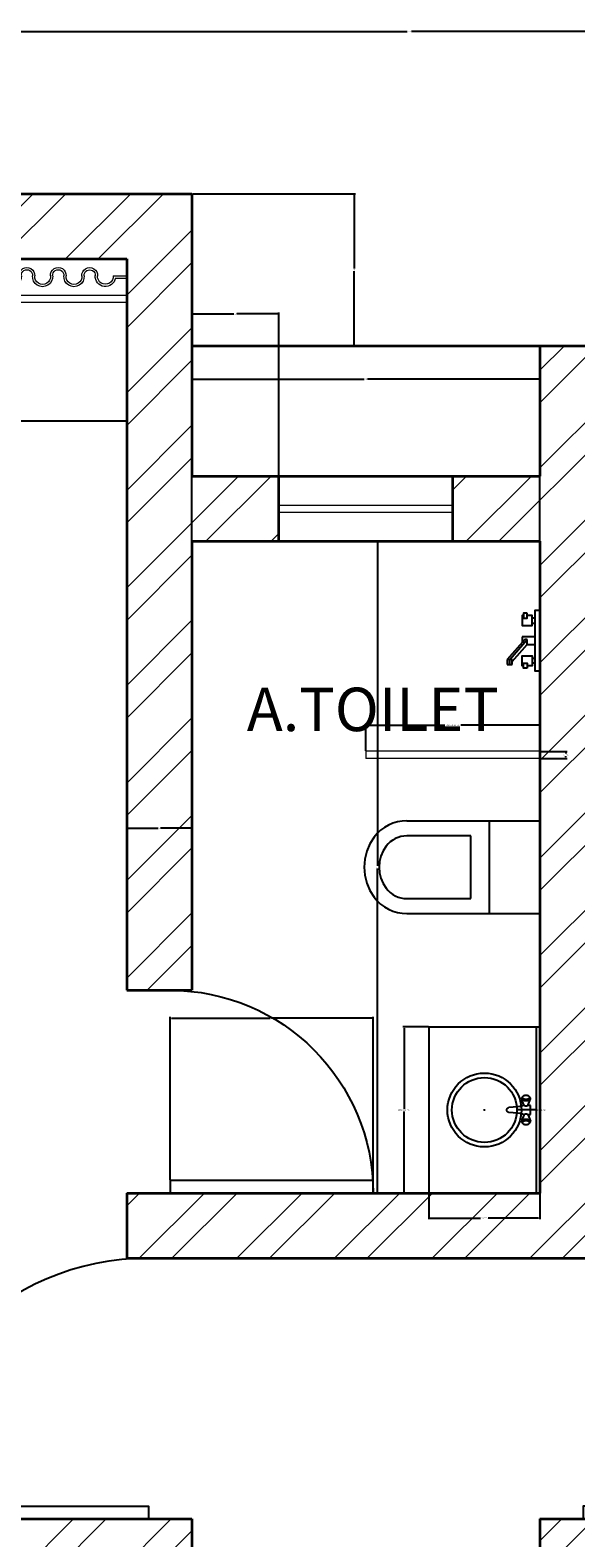
# Model space of a CAD drawing. Units: inches. Extents: x 3449 to 3843, y 1566 to 2054.
# Tile 7 of 8: x 3594 to 3669, y 1846 to 2054. Entities that reach past the tile are written whole.
import ezdxf

# ---------------------------------------------------------------- set-up
doc = ezdxf.new("R2010")
doc.units = ezdxf.units.IN
for name, color, linetype, lineweight in [('A-ANNO-DIMS', 2, 'Continuous', 18), ('A-AREA-IDEN', 7, 'Continuous', 25), ('A-DOOR', 4, 'Continuous', 25), ('A-FURN-DRAP', 32, 'Continuous', 13), ('A-GLAZ', 5, 'Continuous', 18), ('A-WALL', 7, 'Continuous', 35), ('A-WALL-PATT', 251, 'Continuous', 13), ('Сантехника', 7, 'Continuous', 18)]:
    doc.layers.add(name, color=color, linetype=linetype, lineweight=lineweight)
doc.layers.add('SANTEH', color=7, linetype='Continuous')
doc.styles.get("Standard").update_dxf_attribs({"font": 'arial.ttf'})
doc.dimstyles.get("Standard").update_dxf_attribs({"dimtxt": 0.18, "dimasz": 0.18, "dimexe": 0.18, "dimexo": 0.0625, "dimgap": 0.09, "dimtad": 0, "dimtih": 1, "dimtoh": 1, "dimdec": 4, "dimzin": 0, "dimdsep": 46, "dimtxsty": 'Standard', "dimcen": 0.09, "dimadec": 0, "dimazin": 0, "dimtfac": 1, "dimtdec": 4, "dimtofl": 0, "dimtmove": 0, "dimatfit": 3, "dimfxl": 1, "dimtolj": 1, "dimtzin": 0, "dimarcsym": 0})

# ---------------------------------------------------------------- blocks, each defined once
blk = doc.blocks.new('*U5')
for p, q in [((0, 0), (0, -6)), ((36, 0), (36, -6))]:
    blk.add_line(p, q)
blk.add_lwpolyline([(0, 0), (0, 36), (1.75, 36), (1.75, 0)], close=True)
blk.add_arc((0, 0), 36, 0, 90)
blk = doc.blocks.new('*U7')
for p, q in [((0, 0), (0, -6)), ((28, 0), (28, -6))]:
    blk.add_line(p, q)
blk.add_lwpolyline([(0, 0), (0, 28), (1.75, 28), (1.75, 0)], close=True)
blk.add_arc((0, 0), 28, 0, 90)
blk = doc.blocks.new('Basin Built-In Circle_74')
at = {"layer": 'SANTEH'}
for p, q in [((0, 600), (900, 600)), ((0, 0), (0, 600)), ((0, 580), (900, 580)), ((900, 0), (900, 600)), ((371.7, 528.5), (371.5, 525)), ((371.7, 528.5), (371.5, 525)), ((371.5, 525), (371.7, 521.5)), ((371.5, 525), (371.7, 521.5)), ((372.1, 531.8), (371.7, 528.5)), ((372.1, 531.8), (371.7, 528.5)), ((371.7, 521.5), (372.1, 518.2)), ((371.7, 521.5), (372.1, 518.2)), ((372.8, 535), (372.1, 531.8)), ((372.8, 535), (372.1, 531.8)), ((372.1, 518.2), (372.8, 515)), ((372.1, 518.2), (372.8, 515)), ((373.8, 537.9), (372.8, 535)), ((373.8, 537.9), (372.8, 535)), ((372.8, 515), (373.8, 512.1)), ((372.8, 515), (373.8, 512.1)), ((375.1, 540.3), (373.8, 537.9)), ((375.1, 540.3), (373.8, 537.9)), ((373.8, 512.1), (375.1, 509.7)), ((373.8, 512.1), (375.1, 509.7)), ((376.5, 542.3), (375.1, 540.3)), ((376.5, 542.3), (375.1, 540.3)), ((375.1, 509.7), (376.5, 507.7)), ((375.1, 509.7), (376.5, 507.7)), ((378.1, 543.8), (376.5, 542.3)), ((378.1, 543.8), (376.5, 542.3)), ((376.5, 507.7), (378.1, 506.2)), ((376.5, 507.7), (378.1, 506.2)), ((382.6, 547.6), (378.1, 543.8)), ((382.6, 547.6), (378.1, 543.8)), ((379.8, 544.7), (378.1, 543.8)), ((379.8, 544.7), (378.1, 543.8)), ((378.1, 506.2), (379.8, 505.3)), ((382.6, 502.4), (378.1, 506.2)), ((378.1, 506.2), (379.8, 505.3)), ((382.6, 502.4), (378.1, 506.2)), ((381.5, 545), (379.8, 544.7)), ((381.5, 545), (379.8, 544.7)), ((379.8, 505.3), (381.5, 505)), ((379.8, 505.3), (381.5, 505)), ((383.2, 544.7), (381.5, 545)), ((383.2, 544.7), (381.5, 545)), ((381.5, 505), (383.2, 505.3)), ((381.5, 505), (383.2, 505.3)), ((384.6, 548.6), (382.6, 547.6)), ((384.6, 548.6), (382.6, 547.6)), ((382.6, 502.4), (384.6, 501.4)), ((382.6, 502.4), (384.6, 501.4)), ((384.9, 543.8), (383.2, 544.7)), ((384.9, 543.8), (383.2, 544.7)), ((383.2, 505.3), (384.9, 506.2)), ((383.2, 505.3), (384.9, 506.2)), ((386.7, 549), (384.6, 548.6)), ((386.7, 549), (384.6, 548.6)), ((384.6, 501.4), (386.7, 501)), ((384.6, 501.4), (386.7, 501)), ((386.5, 542.3), (384.9, 543.8)), ((386.5, 542.3), (384.9, 543.8)), ((384.9, 506.2), (386.5, 507.7)), ((384.9, 506.2), (386.5, 507.7)), ((387.9, 540.3), (386.5, 542.3)), ((387.9, 540.3), (386.5, 542.3)), ((386.5, 507.7), (387.9, 509.7)), ((386.5, 507.7), (387.9, 509.7)), ((388.8, 548.6), (386.7, 549)), ((388.8, 548.6), (386.7, 549)), ((386.7, 501), (388.8, 501.4)), ((386.7, 501), (388.8, 501.4)), ((389.2, 537.9), (387.9, 540.3)), ((389.2, 537.9), (387.9, 540.3)), ((387.9, 509.7), (389.2, 512.1)), ((387.9, 509.7), (389.2, 512.1)), ((390.8, 547.6), (388.8, 548.6)), ((422.4, 536.8), (388.8, 548.6)), ((390.8, 547.6), (388.8, 548.6)), ((422.4, 536.8), (388.8, 548.6)), ((422.4, 513.2), (388.8, 501.4)), ((422.4, 513.2), (388.8, 501.4)), ((388.8, 501.4), (390.8, 502.4)), ((388.8, 501.4), (390.8, 502.4)), ((390.2, 535), (389.2, 537.9)), ((390.2, 535), (389.2, 537.9)), ((389.2, 512.1), (390.2, 515)), ((389.2, 512.1), (390.2, 515)), ((390.9, 531.8), (390.2, 535)), ((390.9, 531.8), (390.2, 535)), ((390.2, 515), (390.9, 518.2)), ((390.2, 515), (390.9, 518.2)), ((392.7, 545.8), (390.8, 547.6)), ((392.7, 545.8), (390.8, 547.6)), ((390.8, 502.4), (392.7, 504.2)), ((390.8, 502.4), (392.7, 504.2)), ((391.4, 528.5), (390.9, 531.8)), ((391.4, 528.5), (390.9, 531.8)), ((390.9, 518.2), (391.4, 521.5)), ((390.9, 518.2), (391.4, 521.5)), ((391.5, 525), (391.4, 528.5)), ((391.5, 525), (391.4, 528.5)), ((391.4, 521.5), (391.5, 525)), ((391.4, 521.5), (391.5, 525)), ((394.4, 543.4), (392.7, 545.8)), ((394.4, 543.4), (392.7, 545.8)), ((392.7, 504.2), (394.4, 506.6)), ((392.7, 504.2), (394.4, 506.6)), ((395.9, 540.4), (394.4, 543.4)), ((395.9, 540.4), (394.4, 543.4)), ((394.4, 506.6), (395.9, 509.6)), ((394.4, 506.6), (395.9, 509.6)), ((397.1, 537), (395.9, 540.4)), ((397.1, 537), (395.9, 540.4)), ((395.9, 509.6), (397.1, 513)), ((395.9, 509.6), (397.1, 513)), ((398, 533.2), (397.1, 537)), ((398, 533.2), (397.1, 537)), ((397.1, 513), (398, 516.8)), ((397.1, 513), (398, 516.8)), ((398.5, 529.2), (398, 533.2)), ((398.5, 529.2), (398, 533.2)), ((398, 516.8), (398.5, 520.8)), ((398, 516.8), (398.5, 520.8)), ((398.7, 525), (398.5, 529.2)), ((398.7, 525), (398.5, 529.2)), ((398.5, 520.8), (398.7, 525)), ((398.5, 520.8), (398.7, 525)), ((423.4, 536.3), (422.4, 536.8)), ((423.4, 536.3), (422.4, 536.8)), ((422.4, 513.2), (423.4, 513.7)), ((422.4, 513.2), (423.4, 513.7)), ((424.3, 535.4), (423.4, 536.3)), ((424.3, 535.4), (423.4, 536.3)), ((423.4, 513.7), (424.3, 514.6)), ((423.4, 513.7), (424.3, 514.6)), ((425.2, 534.2), (424.3, 535.4)), ((425.2, 534.2), (424.3, 535.4)), ((424.3, 514.6), (425.2, 515.8)), ((424.3, 514.6), (425.2, 515.8)), ((426.7, 535), (424.6, 535)), ((426.7, 535), (424.6, 535)), ((427.1, 515), (424.6, 515)), ((427.1, 515), (424.6, 515)), ((425.2, 548), (425, 547.5)), ((425.2, 548), (425, 547.5)), ((425, 547.5), (425, 547)), ((425, 547.5), (425, 547)), ((425, 547), (425, 535)), ((425, 547), (425, 535)), ((425, 515), (425, 513)), ((425, 515), (425, 513)), ((425, 513), (425, 512.5)), ((425, 513), (425, 512.5)), ((425, 512.5), (425.2, 512)), ((425, 512.5), (425.2, 512)), ((425.4, 548.5), (425.2, 548)), ((425.4, 548.5), (425.2, 548)), ((425.9, 532.7), (425.2, 534.2)), ((425.9, 532.7), (425.2, 534.2)), ((425.2, 515.8), (425.9, 517.3)), ((425.2, 515.8), (425.9, 517.3)), ((425.2, 512), (428.1, 505.1)), ((425.2, 512), (428.1, 505.1)), ((425.7, 548.9), (425.4, 548.5)), ((425.7, 548.9), (425.4, 548.5)), ((426.1, 549.3), (425.7, 548.9)), ((426.1, 549.3), (425.7, 548.9)), ((426.5, 531), (425.9, 532.7)), ((426.5, 531), (425.9, 532.7)), ((425.9, 517.3), (426.5, 519)), ((425.9, 517.3), (426.5, 519)), ((426.5, 549.6), (426.1, 549.3)), ((426.5, 549.6), (426.1, 549.3)), ((427, 549.8), (426.5, 549.6)), ((427, 549.8), (426.5, 549.6)), ((427, 529.1), (426.5, 531)), ((427, 529.1), (426.5, 531)), ((426.5, 519), (427, 520.9)), ((426.5, 519), (427, 520.9)), ((427.5, 550), (427, 549.8)), ((427.5, 550), (427, 549.8)), ((427.2, 527.1), (427, 529.1)), ((427.2, 527.1), (427, 529.1)), ((427, 520.9), (427.2, 522.9)), ((427, 520.9), (427.2, 522.9)), ((427.3, 525), (427.2, 527.1)), ((427.3, 525), (427.2, 527.1)), ((427.2, 522.9), (427.3, 525)), ((427.2, 522.9), (427.3, 525)), ((428, 550), (427.5, 550)), ((428, 550), (427.5, 550)), ((472, 550), (428, 550)), ((472, 550), (428, 550)), ((428, 505.4), (430.7, 493.4)), ((428, 505.4), (430.7, 493.4)), ((430.7, 493.4), (433, 477.1)), ((430.7, 493.4), (433, 477.1)), ((469.3, 493.4), (467, 477.1)), ((469.3, 493.4), (467, 477.1)), ((472, 505.4), (469.3, 493.4)), ((472, 505.4), (469.3, 493.4)), ((474.8, 512), (471.9, 505.1)), ((474.8, 512), (471.9, 505.1)), ((472.5, 550), (472, 550)), ((472.5, 550), (472, 550)), ((473, 549.8), (472.5, 550)), ((473, 549.8), (472.5, 550)), ((472.8, 527.1), (472.7, 525)), ((472.8, 527.1), (472.7, 525)), ((472.7, 525), (472.8, 522.9)), ((472.7, 525), (472.8, 522.9)), ((473, 529.1), (472.8, 527.1)), ((473, 529.1), (472.8, 527.1)), ((472.8, 522.9), (473, 520.9)), ((472.8, 522.9), (473, 520.9)), ((473.5, 549.6), (473, 549.8)), ((473.5, 549.6), (473, 549.8)), ((473.5, 531), (473, 529.1)), ((473.5, 531), (473, 529.1)), ((473, 520.9), (473.5, 519)), ((473, 520.9), (473.5, 519)), ((475.4, 515), (473.2, 515)), ((475.4, 515), (473.2, 515)), ((473.9, 549.3), (473.5, 549.6)), ((473.9, 549.3), (473.5, 549.6)), ((475.4, 535), (473.5, 535)), ((475.4, 535), (473.5, 535)), ((474.1, 532.7), (473.5, 531)), ((474.1, 532.7), (473.5, 531)), ((473.5, 519), (474.1, 517.3)), ((473.5, 519), (474.1, 517.3)), ((474.3, 548.9), (473.9, 549.3)), ((474.3, 548.9), (473.9, 549.3)), ((474.8, 534.2), (474.1, 532.7)), ((474.8, 534.2), (474.1, 532.7)), ((474.1, 517.3), (474.8, 515.8)), ((474.1, 517.3), (474.8, 515.8)), ((474.6, 548.5), (474.3, 548.9)), ((474.6, 548.5), (474.3, 548.9)), ((474.8, 548), (474.6, 548.5)), ((474.8, 548), (474.6, 548.5)), ((475, 547.5), (474.8, 548)), ((475, 547.5), (474.8, 548)), ((475.7, 535.4), (474.8, 534.2)), ((475.7, 535.4), (474.8, 534.2)), ((474.8, 515.8), (475.7, 514.6)), ((474.8, 515.8), (475.7, 514.6)), ((474.8, 512), (475, 512.5)), ((474.8, 512), (475, 512.5)), ((475, 547), (475, 547.5)), ((475, 547), (475, 547.5)), ((475, 535), (475, 547)), ((475, 535), (475, 547)), ((475, 513), (475, 515)), ((475, 513), (475, 515)), ((475, 512.5), (475, 513)), ((475, 512.5), (475, 513)), ((476.6, 536.3), (475.7, 535.4)), ((476.6, 536.3), (475.7, 535.4)), ((475.7, 514.6), (476.6, 513.7)), ((475.7, 514.6), (476.6, 513.7)), ((477.6, 536.8), (476.6, 536.3)), ((477.6, 536.8), (476.6, 536.3)), ((476.6, 513.7), (477.6, 513.2)), ((476.6, 513.7), (477.6, 513.2)), ((477.6, 536.8), (511.2, 548.6)), ((477.6, 536.8), (511.2, 548.6)), ((477.6, 513.2), (511.2, 501.4)), ((477.6, 513.2), (511.2, 501.4)), ((501.5, 529.2), (501.3, 525)), ((501.5, 529.2), (501.3, 525)), ((501.3, 525), (501.5, 520.8)), ((501.3, 525), (501.5, 520.8)), ((502, 533.2), (501.5, 529.2)), ((502, 533.2), (501.5, 529.2)), ((501.5, 520.8), (502, 516.8)), ((501.5, 520.8), (502, 516.8)), ((502.9, 537), (502, 533.2)), ((502.9, 537), (502, 533.2)), ((502, 516.8), (502.9, 513)), ((502, 516.8), (502.9, 513)), ((504.1, 540.4), (502.9, 537)), ((504.1, 540.4), (502.9, 537)), ((502.9, 513), (504.1, 509.6)), ((502.9, 513), (504.1, 509.6)), ((505.6, 543.4), (504.1, 540.4)), ((505.6, 543.4), (504.1, 540.4)), ((504.1, 509.6), (505.6, 506.6)), ((504.1, 509.6), (505.6, 506.6)), ((507.3, 545.8), (505.6, 543.4)), ((507.3, 545.8), (505.6, 543.4)), ((505.6, 506.6), (507.3, 504.2)), ((505.6, 506.6), (507.3, 504.2)), ((509.2, 547.6), (507.3, 545.8)), ((509.2, 547.6), (507.3, 545.8)), ((507.3, 504.2), (509.2, 502.4)), ((507.3, 504.2), (509.2, 502.4)), ((508.6, 528.5), (508.5, 525)), ((508.6, 528.5), (508.5, 525)), ((508.5, 525), (508.6, 521.5)), ((508.5, 525), (508.6, 521.5)), ((509.1, 531.8), (508.6, 528.5)), ((509.1, 531.8), (508.6, 528.5)), ((508.6, 521.5), (509.1, 518.2)), ((508.6, 521.5), (509.1, 518.2)), ((509.8, 535), (509.1, 531.8)), ((509.8, 535), (509.1, 531.8)), ((509.1, 518.2), (509.8, 515)), ((509.1, 518.2), (509.8, 515)), ((511.2, 548.6), (509.2, 547.6)), ((511.2, 548.6), (509.2, 547.6)), ((509.2, 502.4), (511.2, 501.4)), ((509.2, 502.4), (511.2, 501.4)), ((510.8, 537.9), (509.8, 535)), ((510.8, 537.9), (509.8, 535)), ((509.8, 515), (510.8, 512.1)), ((509.8, 515), (510.8, 512.1)), ((512.1, 540.3), (510.8, 537.9)), ((512.1, 540.3), (510.8, 537.9)), ((510.8, 512.1), (512.1, 509.7)), ((510.8, 512.1), (512.1, 509.7)), ((513.3, 549), (511.2, 548.6)), ((513.3, 549), (511.2, 548.6)), ((511.2, 501.4), (513.3, 501)), ((511.2, 501.4), (513.3, 501)), ((513.5, 542.3), (512.1, 540.3)), ((513.5, 542.3), (512.1, 540.3)), ((512.1, 509.7), (513.5, 507.7)), ((512.1, 509.7), (513.5, 507.7)), ((515.4, 548.6), (513.3, 549)), ((515.4, 548.6), (513.3, 549)), ((513.3, 501), (515.4, 501.4)), ((513.3, 501), (515.4, 501.4)), ((515.1, 543.8), (513.5, 542.3)), ((515.1, 543.8), (513.5, 542.3)), ((513.5, 507.7), (515.1, 506.2)), ((513.5, 507.7), (515.1, 506.2)), ((516.8, 544.7), (515.1, 543.8)), ((516.8, 544.7), (515.1, 543.8)), ((515.1, 506.2), (516.8, 505.3)), ((515.1, 506.2), (516.8, 505.3)), ((517.4, 547.6), (515.4, 548.6)), ((517.4, 547.6), (515.4, 548.6)), ((515.4, 501.4), (517.4, 502.4)), ((515.4, 501.4), (517.4, 502.4)), ((518.5, 545), (516.8, 544.7)), ((518.5, 545), (516.8, 544.7)), ((516.8, 505.3), (518.5, 505)), ((516.8, 505.3), (518.5, 505)), ((517.4, 547.6), (521.9, 543.8)), ((517.4, 547.6), (521.9, 543.8)), ((517.4, 502.4), (521.9, 506.2)), ((517.4, 502.4), (521.9, 506.2)), ((520.2, 544.7), (518.5, 545)), ((520.2, 544.7), (518.5, 545)), ((518.5, 505), (520.2, 505.3)), ((518.5, 505), (520.2, 505.3)), ((521.9, 543.8), (520.2, 544.7)), ((521.9, 543.8), (520.2, 544.7)), ((520.2, 505.3), (521.9, 506.2)), ((520.2, 505.3), (521.9, 506.2)), ((523.5, 542.3), (521.9, 543.8)), ((523.5, 542.3), (521.9, 543.8)), ((521.9, 506.2), (523.5, 507.7)), ((521.9, 506.2), (523.5, 507.7)), ((524.9, 540.3), (523.5, 542.3)), ((524.9, 540.3), (523.5, 542.3)), ((523.5, 507.7), (524.9, 509.7)), ((523.5, 507.7), (524.9, 509.7)), ((526.2, 537.9), (524.9, 540.3)), ((526.2, 537.9), (524.9, 540.3)), ((524.9, 509.7), (526.2, 512.1)), ((524.9, 509.7), (526.2, 512.1)), ((527.2, 535), (526.2, 537.9)), ((527.2, 535), (526.2, 537.9)), ((526.2, 512.1), (527.2, 515)), ((526.2, 512.1), (527.2, 515)), ((527.9, 531.8), (527.2, 535)), ((527.9, 531.8), (527.2, 535)), ((527.2, 515), (527.9, 518.2)), ((527.2, 515), (527.9, 518.2)), ((528.3, 528.5), (527.9, 531.8)), ((528.3, 528.5), (527.9, 531.8)), ((527.9, 518.2), (528.3, 521.5)), ((527.9, 518.2), (528.3, 521.5)), ((528.5, 525), (528.3, 528.5)), ((528.5, 525), (528.3, 528.5)), ((528.3, 521.5), (528.5, 525)), ((528.3, 521.5), (528.5, 525)), ((433, 477.2), (435, 456.1)), ((433, 477.2), (435, 456.1)), ((435, 456.1), (436.8, 432.9)), ((435, 456.1), (436.8, 432.9)), ((437, 430.8), (436.8, 432.9)), ((437, 430.8), (436.8, 432.9)), ((437, 430.7), (437, 430.8)), ((437, 430.7), (437, 430.8)), ((437.6, 428.7), (437, 430.7)), ((437.6, 428.7), (437, 430.7)), ((438.6, 426.9), (437.6, 428.7)), ((438.6, 426.9), (437.6, 428.7)), ((440, 425.1), (438.6, 426.9)), ((440, 425.1), (438.6, 426.9)), ((441.6, 423.7), (440, 425.1)), ((441.6, 423.7), (440, 425.1)), ((443.5, 422.5), (441.6, 423.7)), ((443.5, 422.5), (441.6, 423.7)), ((445.6, 421.7), (443.5, 422.5)), ((445.6, 421.7), (443.5, 422.5)), ((445, 421.7), (443.9, 422.4)), ((446.6, 421), (445, 421.7)), ((447.7, 421.2), (445.6, 421.7)), ((447.7, 421.2), (445.6, 421.7)), ((448.3, 420.6), (446.6, 421)), ((450, 421), (447.7, 421.2)), ((450, 421), (447.7, 421.2)), ((450, 420.5), (448.3, 420.6)), ((452.3, 421.2), (450, 421)), ((452.3, 421.2), (450, 421)), ((451.7, 420.6), (450, 420.5)), ((453.4, 421), (451.7, 420.6)), ((454.4, 421.7), (452.3, 421.2)), ((454.4, 421.7), (452.3, 421.2)), ((455, 421.7), (453.4, 421)), ((456.5, 422.5), (454.4, 421.7)), ((456.5, 422.5), (454.4, 421.7)), ((456.1, 422.4), (455, 421.7)), ((458.4, 423.7), (456.5, 422.5)), ((458.4, 423.7), (456.5, 422.5)), ((460, 425.1), (458.4, 423.7)), ((460, 425.1), (458.4, 423.7)), ((461.4, 426.9), (460, 425.1)), ((461.4, 426.9), (460, 425.1)), ((462.4, 428.7), (461.4, 426.9)), ((462.4, 428.7), (461.4, 426.9)), ((463, 430.7), (462.4, 428.7)), ((463, 430.7), (462.4, 428.7)), ((463.2, 432.9), (463, 430.8)), ((463.2, 432.9), (463, 430.8)), ((463, 430.7), (463, 430.8)), ((463, 430.7), (463, 430.8)), ((465, 456.1), (463.2, 432.9)), ((465, 456.1), (463.2, 432.9)), ((467, 477.2), (465, 456.1)), ((467, 477.2), (465, 456.1)), ((0, 0), (900, 0))]:
    blk.add_line(p, q, dxfattribs=at)
for radius in [200, 175.8]:
    blk.add_circle((450, 300), radius, dxfattribs=at)
blk = doc.blocks.new('WC With Cistern_103')
at = {"layer": 'SANTEH'}
for p, q in [((0, 170), (0, 700)), ((370, 700), (0, 700)), ((370, 170), (370, 700)), ((370, 500), (0, 500)), ((60, 425), (60, 170)), ((310, 425), (60, 425)), ((310, 170), (310, 425))]:
    blk.add_line(p, q, dxfattribs=at)
for points in [[(0, 170), (1.1, 151.2), (4.3, 132.7), (9.7, 114.6), (17.1, 97.3), (26.5, 81), (37.7, 65.9), (50.6, 52.1), (65, 40)], [(60, 170), (60.7, 158.1), (62.7, 146.5), (66.1, 135.1), (70.8, 124.2), (76.7, 113.9), (83.8, 104.3), (91.9, 95.7), (101, 88)], [(269, 88), (278.1, 95.7), (286.2, 104.3), (293.3, 113.9), (299.2, 124.2), (303.9, 135.1), (307.3, 146.5), (309.3, 158.1), (310, 170)], [(305, 40), (319.4, 52.1), (332.3, 65.9), (343.5, 81), (352.9, 97.3), (360.3, 114.6), (365.7, 132.7), (368.9, 151.2), (370, 170)], [(101, 88), (120, 76), (140.7, 67.2), (162.6, 61.8), (185, 60), (207.4, 61.8), (229.3, 67.2), (250, 76), (269, 88)], [(65, 40), (92.2, 22.8), (121.8, 10.3), (153, 2.6), (185, 0), (217, 2.6), (248.2, 10.3), (277.8, 22.8), (305, 40)]]:
    blk.add_lwpolyline(points, dxfattribs=at)
blk = doc.blocks.new('Faucet - kit sink front')
at = {"layer": 'SANTEH'}
for p, q in [((-0.25, 3), (3.75, 6.5)), ((3.75, 6), (3.75, 6.5)), ((3.75, 6.5), (4.75, 6.5)), ((4.75, 6.5), (4.75, 6)), ((-0.75, 3.5), (0.3192, 3.5)), ((-0.75, 1), (-0.75, 3.5)), ((3.75, 6), (-0.25, 2.5)), ((4.1921, 5.5041), (0.75, 2.5)), ((3.75, 5.5), (3.75, 6)), ((4.75, 6), (3.75, 6)), ((4.75, 5.5), (3.75, 5.5)), ((4.75, 6), (4.75, 5.5)), ((-4.5, 1), (-4.5, 1.5)), ((-3.5, 1.5), (-3.5, 1)), ((-0.25, 2.5), (-0.25, 3)), ((0.75, 2.5), (-0.25, 2.5)), ((0.75, 2.5), (0.75, 1)), ((3.5, 1.5), (3.5, 1)), ((4.5, 1), (4.5, 1.5))]:
    blk.add_line(p, q, dxfattribs=at)
for points in [[(-5.5, 2.5), (-5.5, 3.25), (-4.5, 3.25), (-4.5, 2.5)], [(5.5, 2.5), (5.5, 3.25), (4.5, 3.25), (4.5, 2.5)], [(-6, 0), (-6, 1), (6, 1), (6, 0)]]:
    blk.add_lwpolyline(points, close=True, dxfattribs=at)
for points in [[(-5, 3.2513), (-5, 3.5), (-3, 3.5), (-3, 1.5), (-5, 1.5), (-5, 2.5)], [(5, 3.2513), (5, 3.5), (3, 3.5), (3, 1.5), (5, 1.5), (5, 2.5)]]:
    blk.add_lwpolyline(points, dxfattribs=at)
blk = doc.blocks.new('DRAPERY-PANEL')
for p, q in [((1.19, 47.95), (1.19, 49.52)), ((1.5, 47.66), (1.5, 49.52))]:
    blk.add_line(p, q)
for centre, radius, start, end in [((1.42, 46.57), 1.4, 99.481, 274.2422), ((1.42, 46.57), 1.09, 85.7578, 274.2422), ((1.55, 44.41), 1.09, 265.7578, 94.2422), ((1.55, 44.41), 0.776, 265.7578, 94.2422), ((1.4, 42.24), 1.4, 85.7578, 274.2422), ((1.4, 42.24), 1.09, 85.7578, 274.2422), ((1.56, 40.07), 1.09, 265.7578, 94.2422), ((1.56, 40.07), 0.776, 265.7578, 94.2422), ((1.4, 37.91), 1.4, 85.7578, 274.2422), ((1.4, 37.91), 1.09, 85.7578, 274.2422), ((1.56, 35.74), 1.09, 265.7578, 94.2422), ((1.56, 35.74), 0.776, 265.7578, 94.2422), ((1.4, 33.58), 1.4, 85.7578, 274.2422), ((1.4, 33.58), 1.09, 85.7578, 274.2422), ((1.56, 31.41), 1.09, 265.7578, 94.2422), ((1.56, 31.41), 0.776, 265.7578, 94.2422), ((1.41, 29.24), 1.4, 85.7578, 274.2422), ((1.41, 29.24), 1.09, 85.7578, 274.2422), ((1.57, 27.08), 1.09, 265.7578, 94.2422), ((1.57, 27.08), 0.776, 265.7578, 94.2422), ((1.41, 24.91), 1.4, 85.7578, 274.2422), ((1.41, 24.91), 1.09, 85.7578, 274.2422), ((1.57, 22.74), 1.09, 265.7578, 94.2422), ((1.57, 22.74), 0.776, 265.7578, 94.2422), ((1.41, 20.58), 1.4, 85.7578, 274.2422), ((1.41, 20.58), 1.09, 85.7578, 274.2422), ((1.58, 18.41), 1.09, 265.7578, 94.2422), ((1.58, 18.41), 0.776, 265.7578, 94.2422), ((1.42, 16.25), 1.4, 85.7578, 274.2422), ((1.42, 16.25), 1.09, 85.7578, 274.2422), ((1.58, 14.08), 1.09, 265.7578, 94.2422), ((1.58, 14.08), 0.776, 265.7578, 94.2422), ((1.42, 11.91), 1.4, 85.7578, 274.2422), ((1.42, 11.91), 1.09, 85.7578, 274.2422), ((1.58, 9.75), 1.09, 265.7578, 94.2422), ((1.58, 9.75), 0.776, 265.7578, 94.2422), ((1.43, 7.58), 1.4, 85.7578, 274.2422), ((1.43, 7.58), 1.09, 85.7578, 274.2422), ((1.59, 5.42), 1.09, 265.7578, 94.2422), ((1.43, 3.25), 1.4, 85.7578, 274.2422), ((1.43, 3.25), 1.09, 85.7578, 274.2422), ((1.59, 5.42), 0.776, 265.7578, 94.2422), ((1.59, 1.08), 1.09, 265.7578, 94.2422), ((1.59, 1.08), 0.776, 265.7578, 94.2422)]:
    blk.add_arc(centre, radius, start, end)
blk = doc.blocks.new('SHOWER-SCREEN-24')
for p, q in [((0, 24), (0, 0)), ((1, 24), (1, 0)), ((0, 0), (1, 0))]:
    blk.add_line(p, q)
blk = doc.blocks.new('GLAZING-24')
for p, q in [((24, 1), (0, 1)), ((24, 0), (0, 0))]:
    blk.add_line(p, q)
blk = doc.blocks.new('*D48')
at = {"layer": 'A-ANNO-DIMS', "color": 0, "lineweight": -2, "transparency": 16777216}
for p, q in [((3648.73, 1916.56), (3645.17, 1916.56)), ((3645.35, 1916.38), (3645.35, 1905.27)), ((3645.35, 1893.79), (3645.35, 1904.9)), ((3648.73, 1893.61), (3645.17, 1893.61))]:
    blk.add_line(p, q, dxfattribs=at)
at = {"layer": 'A-ANNO-DIMS', "color": 0, "transparency": 16777216}
for points in [[(3645.32, 1916.38), (3645.38, 1916.38), (3645.35, 1916.56)], [(3645.32, 1893.79), (3645.38, 1893.79), (3645.35, 1893.61)]]:
    blk.add_solid(points, dxfattribs=at)
at = {"layer": 'Defpoints', "color": 0, "transparency": 16777216}
for p in [(3648.79, 1916.56), (3645.35, 1893.61), (3648.79, 1893.61)]:
    blk.add_point(p, dxfattribs=at)
at = {"layer": 'A-ANNO-DIMS', "color": 0, "transparency": 16777216, "insert": (3645.35, 1905.09), "char_height": 0.18, "attachment_point": 5}
blk.add_mtext('\\A1;BASIN 23 TYP.', dxfattribs=at)
blk = doc.blocks.new('*D49')
at = {"layer": 'A-ANNO-DIMS', "color": 0, "lineweight": -2, "transparency": 16777216}
for p, q in [((3648.79, 1893.55), (3648.79, 1889.99)), ((3664.09, 1893.55), (3664.09, 1889.99)), ((3648.97, 1890.17), (3655.92, 1890.17)), ((3663.91, 1890.17), (3656.96, 1890.17))]:
    blk.add_line(p, q, dxfattribs=at)
at = {"layer": 'A-ANNO-DIMS', "color": 0, "transparency": 16777216}
for points in [[(3648.97, 1890.2), (3648.97, 1890.14), (3648.79, 1890.17)], [(3663.91, 1890.2), (3663.91, 1890.14), (3664.09, 1890.17)]]:
    blk.add_solid(points, dxfattribs=at)
at = {"layer": 'Defpoints', "color": 0, "transparency": 16777216}
for p in [(3648.79, 1893.61), (3664.09, 1893.61), (3664.09, 1890.17)]:
    blk.add_point(p, dxfattribs=at)
at = {"layer": 'A-ANNO-DIMS', "color": 0, "transparency": 16777216, "insert": (3656.44, 1890.17), "char_height": 0.18, "attachment_point": 5}
blk.add_mtext('\\A1;15 TYP.', dxfattribs=at)
blk = doc.blocks.new('*D56')
at = {"layer": 'A-ANNO-DIMS', "color": 0, "lineweight": -2, "transparency": 16777216}
for p, q in [((3640.09, 1954.68), (3640.09, 1958.39)), ((3640.27, 1958.21), (3651, 1958.21)), ((3663.91, 1958.21), (3653.17, 1958.21)), ((3664.09, 1954.68), (3664.09, 1958.39))]:
    blk.add_line(p, q, dxfattribs=at)
at = {"layer": 'A-ANNO-DIMS', "color": 0, "transparency": 16777216}
for points in [[(3640.27, 1958.24), (3640.27, 1958.18), (3640.09, 1958.21)], [(3663.91, 1958.24), (3663.91, 1958.18), (3664.09, 1958.21)]]:
    blk.add_solid(points, dxfattribs=at)
at = {"layer": 'Defpoints', "color": 0, "transparency": 16777216}
for p in [(3664.09, 1958.21), (3640.09, 1954.61), (3664.09, 1954.61)]:
    blk.add_point(p, dxfattribs=at)
at = {"layer": 'A-ANNO-DIMS', "color": 0, "transparency": 16777216, "insert": (3652.09, 1958.21), "char_height": 0.18, "attachment_point": 5}
blk.add_mtext('\\A1;SCREEN 24 TYP.', dxfattribs=at)
blk = doc.blocks.new('*D57')
at = {"layer": 'A-ANNO-DIMS', "color": 0, "lineweight": -2, "transparency": 16777216}
for p, q in [((3664.15, 1954.61), (3667.87, 1954.61)), ((3664.15, 1953.61), (3667.87, 1953.61)), ((3667.69, 1954.43), (3667.69, 1954.29)), ((3667.69, 1953.79), (3667.69, 1953.93))]:
    blk.add_line(p, q, dxfattribs=at)
at = {"layer": 'A-ANNO-DIMS', "color": 0, "transparency": 16777216}
for points in [[(3667.66, 1954.43), (3667.72, 1954.43), (3667.69, 1954.61)], [(3667.66, 1953.79), (3667.72, 1953.79), (3667.69, 1953.61)]]:
    blk.add_solid(points, dxfattribs=at)
at = {"layer": 'Defpoints', "color": 0, "transparency": 16777216}
for p in [(3664.09, 1954.61), (3664.09, 1953.61), (3667.69, 1953.61)]:
    blk.add_point(p, dxfattribs=at)
at = {"layer": 'A-ANNO-DIMS', "color": 0, "transparency": 16777216, "insert": (3667.69, 1954.11), "char_height": 0.18, "attachment_point": 5}
blk.add_mtext('\\A1;1 TYP.', dxfattribs=at)
blk = doc.blocks.new('*D76')
at = {"layer": 'A-ANNO-DIMS', "color": 0, "lineweight": -2, "transparency": 16777216}
for p, q in [((3472.09, 2031.68), (3472.09, 2054.19)), ((3472.27, 2054.01), (3645.8, 2054.01)), ((3819.91, 2054.01), (3646.38, 2054.01)), ((3820.09, 1986.68), (3820.09, 2054.19))]:
    blk.add_line(p, q, dxfattribs=at)
at = {"layer": 'A-ANNO-DIMS', "color": 0, "transparency": 16777216}
for points in [[(3472.27, 2054.04), (3472.27, 2053.98), (3472.09, 2054.01)], [(3819.91, 2054.04), (3819.91, 2053.98), (3820.09, 2054.01)]]:
    blk.add_solid(points, dxfattribs=at)
at = {"layer": 'Defpoints', "color": 0, "transparency": 16777216}
for p in [(3820.09, 2054.01), (3472.09, 2031.61), (3820.09, 1986.61)]:
    blk.add_point(p, dxfattribs=at)
at = {"layer": 'A-ANNO-DIMS', "color": 0, "transparency": 16777216, "insert": (3646.09, 2054.01), "char_height": 0.18, "attachment_point": 5}
blk.add_mtext('\\A1;348', dxfattribs=at)
blk = doc.blocks.new('*D78')
at = {"layer": 'A-ANNO-DIMS', "color": 0, "lineweight": -2, "transparency": 16777216}
for p, q in [((3616.15, 2031.61), (3638.67, 2031.61)), ((3638.49, 2031.43), (3638.49, 2021.29)), ((3638.49, 2010.79), (3638.49, 2020.93)), ((3616.15, 2010.61), (3638.67, 2010.61))]:
    blk.add_line(p, q, dxfattribs=at)
at = {"layer": 'A-ANNO-DIMS', "color": 0, "transparency": 16777216}
for points in [[(3638.46, 2031.43), (3638.52, 2031.43), (3638.49, 2031.61)], [(3638.46, 2010.79), (3638.52, 2010.79), (3638.49, 2010.61)]]:
    blk.add_solid(points, dxfattribs=at)
at = {"layer": 'Defpoints', "color": 0, "transparency": 16777216}
for p in [(3616.09, 2031.61), (3616.09, 2010.61), (3638.49, 2010.61)]:
    blk.add_point(p, dxfattribs=at)
at = {"layer": 'A-ANNO-DIMS', "color": 0, "transparency": 16777216, "insert": (3638.49, 2021.11), "char_height": 0.18, "attachment_point": 5}
blk.add_mtext('\\A1;21', dxfattribs=at)
blk = doc.blocks.new('*D82')
at = {"layer": 'A-ANNO-DIMS', "color": 0, "lineweight": -2, "transparency": 16777216}
for p, q in [((3481.09, 2022.55), (3481.09, 2000.03)), ((3607.09, 2022.55), (3607.09, 2000.03)), ((3481.27, 2000.21), (3543.81, 2000.21)), ((3606.91, 2000.21), (3544.37, 2000.21))]:
    blk.add_line(p, q, dxfattribs=at)
at = {"layer": 'A-ANNO-DIMS', "color": 0, "transparency": 16777216}
for points in [[(3481.27, 2000.24), (3481.27, 2000.18), (3481.09, 2000.21)], [(3606.91, 2000.24), (3606.91, 2000.18), (3607.09, 2000.21)]]:
    blk.add_solid(points, dxfattribs=at)
at = {"layer": 'Defpoints', "color": 0, "transparency": 16777216}
for p in [(3481.09, 2022.61), (3607.09, 2022.61), (3481.09, 2000.21)]:
    blk.add_point(p, dxfattribs=at)
at = {"layer": 'A-ANNO-DIMS', "color": 0, "transparency": 16777216, "insert": (3544.09, 2000.21), "char_height": 0.18, "attachment_point": 5}
blk.add_mtext('\\A1;126', dxfattribs=at)
blk = doc.blocks.new('*D83')
at = {"layer": 'A-ANNO-DIMS', "color": 0, "lineweight": -2, "transparency": 16777216}
for p, q in [((3616.09, 1983.68), (3616.09, 2006.19)), ((3616.27, 2006.01), (3639.87, 2006.01)), ((3663.91, 2006.01), (3640.31, 2006.01)), ((3664.09, 1983.68), (3664.09, 2006.19))]:
    blk.add_line(p, q, dxfattribs=at)
at = {"layer": 'A-ANNO-DIMS', "color": 0, "transparency": 16777216}
for points in [[(3616.27, 2006.04), (3616.27, 2005.98), (3616.09, 2006.01)], [(3663.91, 2006.04), (3663.91, 2005.98), (3664.09, 2006.01)]]:
    blk.add_solid(points, dxfattribs=at)
at = {"layer": 'Defpoints', "color": 0, "transparency": 16777216}
for p in [(3664.09, 2006.01), (3616.09, 1983.61), (3664.09, 1983.61)]:
    blk.add_point(p, dxfattribs=at)
at = {"layer": 'A-ANNO-DIMS', "color": 0, "transparency": 16777216, "insert": (3640.09, 2006.01), "char_height": 0.18, "attachment_point": 5}
blk.add_mtext('\\A1;48', dxfattribs=at)
blk = doc.blocks.new('*D84')
at = {"layer": 'A-ANNO-DIMS', "color": 0, "lineweight": -2, "transparency": 16777216}
for p, q in [((3664.03, 1983.61), (3641.51, 1983.61)), ((3641.69, 1983.43), (3641.69, 1938.8)), ((3641.69, 1893.79), (3641.69, 1938.43)), ((3664.03, 1893.61), (3641.51, 1893.61))]:
    blk.add_line(p, q, dxfattribs=at)
at = {"layer": 'A-ANNO-DIMS', "color": 0, "transparency": 16777216}
for points in [[(3641.66, 1983.43), (3641.72, 1983.43), (3641.69, 1983.61)], [(3641.66, 1893.79), (3641.72, 1893.79), (3641.69, 1893.61)]]:
    blk.add_solid(points, dxfattribs=at)
at = {"layer": 'Defpoints', "color": 0, "transparency": 16777216}
for p in [(3641.69, 1983.61), (3664.09, 1983.61), (3664.09, 1893.61)]:
    blk.add_point(p, dxfattribs=at)
at = {"layer": 'A-ANNO-DIMS', "color": 0, "transparency": 16777216, "insert": (3641.69, 1938.61), "char_height": 0.18, "attachment_point": 5}
blk.add_mtext('\\A1;90', dxfattribs=at)
blk = doc.blocks.new('*D110')
at = {"layer": 'A-ANNO-DIMS', "color": 0, "lineweight": -2, "transparency": 16777216}
for p, q in [((3613.09, 1895.43), (3613.09, 1917.94)), ((3613.27, 1917.76), (3626.87, 1917.76)), ((3640.91, 1917.76), (3627.31, 1917.76)), ((3641.09, 1895.43), (3641.09, 1917.94))]:
    blk.add_line(p, q, dxfattribs=at)
at = {"layer": 'A-ANNO-DIMS', "color": 0, "transparency": 16777216}
for points in [[(3613.27, 1917.79), (3613.27, 1917.73), (3613.09, 1917.76)], [(3640.91, 1917.79), (3640.91, 1917.73), (3641.09, 1917.76)]]:
    blk.add_solid(points, dxfattribs=at)
at = {"layer": 'Defpoints', "color": 0, "transparency": 16777216}
for p in [(3641.09, 1917.76), (3613.09, 1895.36), (3641.09, 1895.36)]:
    blk.add_point(p, dxfattribs=at)
at = {"layer": 'A-ANNO-DIMS', "color": 0, "transparency": 16777216, "insert": (3627.09, 1917.76), "char_height": 0.18, "attachment_point": 5}
blk.add_mtext('\\A1;28', dxfattribs=at)
blk = doc.blocks.new('*D112')
at = {"layer": 'A-ANNO-DIMS', "color": 0, "lineweight": -2, "transparency": 16777216}
for p, q in [((3607.09, 1921.68), (3607.09, 1944.19)), ((3607.27, 1944.01), (3611.44, 1944.01)), ((3615.91, 1944.01), (3611.74, 1944.01)), ((3616.09, 1921.68), (3616.09, 1944.19))]:
    blk.add_line(p, q, dxfattribs=at)
at = {"layer": 'A-ANNO-DIMS', "color": 0, "transparency": 16777216}
for points in [[(3607.27, 1944.04), (3607.27, 1943.98), (3607.09, 1944.01)], [(3615.91, 1944.04), (3615.91, 1943.98), (3616.09, 1944.01)]]:
    blk.add_solid(points, dxfattribs=at)
at = {"layer": 'Defpoints', "color": 0, "transparency": 16777216}
for p in [(3616.09, 1944.01), (3607.09, 1921.61), (3616.09, 1921.61)]:
    blk.add_point(p, dxfattribs=at)
at = {"layer": 'A-ANNO-DIMS', "color": 0, "transparency": 16777216, "insert": (3611.59, 1944.01), "char_height": 0.18, "attachment_point": 5}
blk.add_mtext('\\A1;9', dxfattribs=at)
blk = doc.blocks.new('*D121')
at = {"layer": 'A-ANNO-DIMS', "color": 0, "lineweight": -2, "transparency": 16777216}
for p, q in [((3616.09, 1992.68), (3616.09, 2015.19)), ((3616.27, 2015.01), (3621.88, 2015.01)), ((3627.91, 2015.01), (3622.3, 2015.01)), ((3628.09, 1992.68), (3628.09, 2015.19))]:
    blk.add_line(p, q, dxfattribs=at)
at = {"layer": 'A-ANNO-DIMS', "color": 0, "transparency": 16777216}
for points in [[(3616.27, 2015.04), (3616.27, 2014.98), (3616.09, 2015.01)], [(3627.91, 2015.04), (3627.91, 2014.98), (3628.09, 2015.01)]]:
    blk.add_solid(points, dxfattribs=at)
at = {"layer": 'Defpoints', "color": 0, "transparency": 16777216}
for p in [(3628.09, 2015.01), (3616.09, 1992.61), (3628.09, 1992.61)]:
    blk.add_point(p, dxfattribs=at)
at = {"layer": 'A-ANNO-DIMS', "color": 0, "transparency": 16777216, "insert": (3622.09, 2015.01), "char_height": 0.18, "attachment_point": 5}
blk.add_mtext('\\A1;12', dxfattribs=at)
blk = doc.blocks.new('*D128')
at = {"layer": 'A-ANNO-DIMS', "color": 0, "lineweight": -2, "transparency": 16777216}
for p, q in [((3656.35, 1905.09), (3656.53, 1905.09)), ((3656.44, 1905), (3656.44, 1905.18)), ((3663.61, 1905.09), (3661.1, 1905.09))]:
    blk.add_line(p, q, dxfattribs=at)
at = {"layer": 'A-ANNO-DIMS', "color": 0, "transparency": 16777216}
blk.add_solid([(3661.1, 1905.12), (3661.1, 1905.06), (3660.92, 1905.09)], dxfattribs=at)
at = {"layer": 'Defpoints', "color": 0, "transparency": 16777216}
for p in [(3651.96, 1905.09), (3660.92, 1905.09)]:
    blk.add_point(p, dxfattribs=at)
at = {"layer": 'A-ANNO-DIMS', "color": 0, "transparency": 16777216, "insert": (3664.3, 1905.09), "char_height": 0.18, "attachment_point": 5}
blk.add_mtext('\\A1;2X ∅8.965', dxfattribs=at)

msp = doc.modelspace()

# ---------------------------------------------------------------- hatches: boundary and pattern name
at = {"layer": 'A-WALL-PATT'}
h = msp.add_hatch(dxfattribs=at)
h.set_pattern_fill('ANSI32', color=256)
edge = h.paths.add_edge_path()
edge.add_line((3481.088, 2022.6144), (3508.088, 2022.6144))
edge.add_line((3508.088, 2022.6144), (3508.088, 2031.6144))
edge.add_line((3508.088, 2031.6144), (3472.088, 2031.6144))
edge.add_line((3472.088, 2031.6144), (3472.088, 1779.6144))
edge.add_line((3472.088, 1779.6144), (3481.088, 1779.6144))
edge.add_line((3481.088, 1779.6144), (3481.088, 1839.6144))
edge.add_line((3481.088, 1839.6144), (3571.088, 1839.6144))
edge.add_line((3571.088, 1839.6144), (3571.088, 1824.3194))
edge.add_line((3571.088, 1824.3194), (3571.088, 1821.6144))
edge.add_line((3571.088, 1821.6144), (3580.088, 1821.6144))
edge.add_line((3580.088, 1821.6144), (3580.088, 1825.1908))
edge.add_ellipse((3580.1411, 1825.2442), major_axis=(0, 0.0754), ratio=0.99913951, start_angle=90, end_angle=135.183195, ccw=False)
edge.add_line((3580.0017, 1825.3196), (3580.0658, 1825.3196))
edge.add_line((3580.0658, 1825.3196), (3580.066, 1839.6365))
edge.add_line((3580.066, 1839.6365), (3616.088, 1839.6365))
edge.add_line((3616.088, 1839.6365), (3616.088, 1848.6144))
edge.add_line((3616.088, 1848.6144), (3610.088, 1848.6144))
edge.add_line((3610.088, 1848.6144), (3574.088, 1848.6144))
edge.add_line((3574.088, 1848.6144), (3481.088, 1848.6144))
edge.add_line((3481.088, 1848.6144), (3481.088, 1872.6144))
edge.add_line((3481.088, 1872.6144), (3481.088, 2022.6144))
h.paths.add_polyline_path([(3550.088, 1779.6144), (3616.088, 1779.6144), (3616.088, 1791.6144), (3505.088, 1791.6144), (3505.088, 1779.6144), (3541.088, 1779.6144), (3541.088, 1657.6144), (3481.088, 1657.6144), (3481.088, 1588.6144), (3496.088, 1588.6144), (3496.088, 1594.6144), (3496.088, 1597.6144), (3490.088, 1597.6144), (3490.088, 1648.6144), (3550.088, 1648.6144)])
h.paths.add_polyline_path([(3775.088, 1612.6144), (3766.088, 1612.6144), (3766.088, 1597.6144), (3536.088, 1597.6144), (3536.088, 1588.6144), (3775.088, 1588.6144)])
h.paths.add_polyline_path([(3820.088, 1756.6144), (3811.088, 1756.6144), (3811.088, 1732.6144), (3664.088, 1732.6144), (3664.088, 1723.6144), (3766.088, 1723.6144), (3766.088, 1708.6144), (3775.088, 1708.6144), (3775.088, 1723.6144), (3820.088, 1723.6144)])
h.paths.add_polyline_path([(3820.088, 1986.6144), (3745.088, 1986.6144), (3745.088, 2010.6144), (3664.088, 2010.6144), (3664.088, 1992.6144), (3652.088, 1992.6144), (3652.088, 1983.6144), (3664.088, 1983.6144), (3664.088, 1893.6144), (3648.793, 1893.6144), (3607.088, 1893.6144), (3607.088, 1884.6144), (3673.088, 1884.6144), (3673.088, 2001.6144), (3736.088, 2001.6144), (3736.088, 1977.6144), (3811.088, 1977.6144), (3811.088, 1949.1144), (3820.088, 1949.1144)])
h.paths.add_polyline_path([(3628.088, 1992.6144), (3616.088, 1992.6144), (3616.088, 2031.6144), (3580.088, 2031.6144), (3580.088, 2022.6144), (3607.088, 2022.6144), (3607.088, 1921.6144), (3613.088, 1921.6144), (3616.088, 1921.6144), (3616.088, 1983.6144), (3628.088, 1983.6144)])
h.paths.add_polyline_path([(3820.088, 1877.1144), (3811.088, 1877.1144), (3811.088, 1848.6144), (3664.088, 1848.6144), (3664.088, 1839.6144), (3700.088, 1839.6144), (3811.088, 1839.6144), (3811.088, 1815.6144), (3820.088, 1815.6144)])

# ---------------------------------------------------------------- linework, layer by layer
at = {"layer": 'A-FURN-DRAP'}
for p, q in [((3481.088, 2017.6144), (3607.088, 2017.6144)), ((3481.088, 2016.6144), (3607.088, 2016.6144))]:
    msp.add_line(p, q, dxfattribs=at)
at = {"layer": 'A-WALL'}
for p, q in [((3508.088, 2031.6144), (3616.088, 2031.6144)), ((3616.088, 2031.6144), (3616.088, 1992.6144)), ((3481.088, 2022.6144), (3607.088, 2022.6144)), ((3607.088, 2022.6144), (3607.088, 1921.6144)), ((3616.088, 2010.6144), (3745.088, 2010.6144)), ((3664.088, 2010.6144), (3664.088, 1992.6144)), ((3664.088, 2010.6144), (3745.088, 2010.6144)), ((3616.088, 1992.6144), (3652.088, 1992.6144)), ((3628.088, 1983.6144), (3628.088, 1992.6144)), ((3652.088, 1983.6144), (3652.088, 1992.6144)), ((3652.088, 1992.6144), (3664.088, 1992.6144)), ((3616.088, 1983.6144), (3664.088, 1983.6144)), ((3616.088, 1983.6144), (3616.088, 1921.6144)), ((3664.088, 1983.6144), (3664.088, 1893.6144)), ((3607.088, 1921.6144), (3616.088, 1921.6144)), ((3607.088, 1893.6144), (3664.088, 1893.6144)), ((3607.088, 1893.6144), (3607.088, 1884.6144)), ((3607.088, 1884.6144), (3673.088, 1884.6144)), ((3481.088, 1848.6144), (3616.088, 1848.6144)), ((3616.088, 1848.6144), (3616.088, 1839.6144)), ((3664.088, 1848.6144), (3811.088, 1848.6144)), ((3664.088, 1848.6144), (3664.088, 1839.6144))]:
    msp.add_line(p, q, dxfattribs=at)

# ---------------------------------------------------------------- block references
at = {"layer": 'A-DOOR', "xscale": -1, "rotation": 270}
for name, p in [('*U7', (3613.088, 1893.6144)), ('*U5', (3670.088, 1848.6144))]:
    msp.add_blockref(name, p, dxfattribs=at)
at = {"layer": 'A-DOOR', "rotation": 90}
msp.add_blockref('*U5', (3610.088, 1848.6144), dxfattribs=at)
at = {"layer": 'A-FURN-DRAP', "extrusion": (0, 0, -1), "zscale": -1, "rotation": 89.99999999999226}
msp.add_blockref('DRAPERY-PANEL', (-3557.5696, 2018.7734), dxfattribs=at)
at = {"layer": 'A-GLAZ', "rotation": 180}
msp.add_blockref('GLAZING-24', (3652.088, 1988.6148), dxfattribs=at)
at = {"layer": 'Сантехника'}
for name, p, xscale, yscale, zscale, rotation in [('Faucet - kit sink front', (3664.088, 1969.8979), -0.6928340246039085, 0.6928340246039085, 0.6928340246039085, 90), ('WC With Cistern_103', (3639.8388, 1945.0231), 0.0346417012301954, 0.0346417012301954, 0.0346417012301954, 270)]:
    msp.add_blockref(name, p, dxfattribs=dict(at, xscale=xscale, yscale=yscale, zscale=zscale, rotation=rotation))
at = {"layer": 'Сантехника', "rotation": 270.0000000000025}
msp.add_blockref('SHOWER-SCREEN-24', (3640.0876, 1954.6144), dxfattribs=at)
at = {"layer": 'Сантехника', "ltscale": 5, "xscale": 0.0254916274909978, "yscale": 0.0254916274909978, "zscale": 0.0254916274909978, "rotation": 270}
msp.add_blockref('Basin Built-In Circle_74', (3648.793, 1916.5569), dxfattribs=at)

# ---------------------------------------------------------------- texts
at = {"layer": 'A-AREA-IDEN', "insert": (3623.6446, 1963.4058), "char_height": 6, "attachment_point": 1}
msp.add_mtext_dynamic_manual_height_columns('A.TOILET', width=95.638287, gutter_width=12.5, heights=[0], dxfattribs=at)

# ---------------------------------------------------------------- dimensions: what is measured, and where the dimension line sits
at = {"layer": 'A-ANNO-DIMS'}
for base, p1, p2, picture, middle in [((3820.088, 2054.0144), (3472.088, 2031.6144), (3820.088, 1986.6144), '*D76', (3646.088, 2054.0144)), ((3628.088, 2015.0144), (3616.088, 1992.6144), (3628.088, 1992.6144), '*D121', (3622.088, 2015.0144)), ((3664.088, 2006.0144), (3616.088, 1983.6144), (3664.088, 1983.6144), '*D83', (3640.088, 2006.0144)), ((3616.088, 1944.0144), (3607.088, 1921.6144), (3616.088, 1921.6144), '*D112', (3611.588, 1944.0144)), ((3641.088, 1917.7644), (3613.088, 1895.3644), (3641.088, 1895.3644), '*D110', (3627.088, 1917.7644))]:
    dim = msp.add_linear_dim(base=base, p1=p1, p2=p2, dimstyle='Standard', override={"dimdec": 0, "dimlfac": 1, "dimrnd": 0, "dimzin": 0, "dimdsep": 46, "dimlunit": 2}, dxfattribs=at)
    dim.commit()
    dim.dimension.update_dxf_attribs({"geometry": picture, "text_midpoint": middle})
for base, p1, p2, angle, picture, middle in [((3638.488, 2010.6144), (3616.088, 2031.6144), (3616.088, 2010.6144), 270, '*D78', (3638.488, 2021.1144)), ((3481.088, 2000.2144), (3607.088, 2022.6144), (3481.088, 2022.6144), 180, '*D82', (3544.088, 2000.2144)), ((3641.688, 1983.6144), (3664.088, 1893.6144), (3664.088, 1983.6144), 90, '*D84', (3641.688, 1938.6144))]:
    dim = msp.add_linear_dim(base=base, p1=p1, p2=p2, angle=angle, dimstyle='Standard', override={"dimdec": 0, "dimlfac": 1, "dimrnd": 0, "dimzin": 0, "dimdsep": 46, "dimlunit": 2}, dxfattribs=at)
    dim.commit()
    dim.dimension.update_dxf_attribs({"geometry": picture, "text_midpoint": middle})
for base, p1, p2, angle, text, picture, middle in [((3664.088, 1958.2144), (3640.088, 1954.6144), (3664.088, 1954.6144), 0, 'SCREEN <> TYP.', '*D56', (3652.088, 1958.2144)), ((3667.688, 1953.6144), (3664.088, 1954.6144), (3664.088, 1953.6144), 270, '<> TYP.', '*D57', (3667.688, 1954.1144)), ((3645.3517, 1893.6144), (3648.793, 1916.5569), (3648.793, 1893.6144), 270, 'BASIN <> TYP.', '*D48', (3645.3517, 1905.0856))]:
    dim = msp.add_linear_dim(base=base, p1=p1, p2=p2, angle=angle, text=text, dimstyle='Standard', override={"dimdec": 0, "dimlfac": 1, "dimrnd": 0, "dimzin": 0, "dimdsep": 46, "dimlunit": 2}, dxfattribs=at)
    dim.commit()
    dim.dimension.update_dxf_attribs({"geometry": picture, "text_midpoint": middle})
dim = msp.add_diameter_dim_2p(p1=(3651.958, 1905.0853), p2=(3660.9231, 1905.086), text='2X <>', dimstyle='Standard', override={"dimdec": 3, "dimlfac": 1, "dimrnd": 0, "dimzin": 0, "dimdsep": 46, "dimlunit": 2}, dxfattribs=at)
dim.commit()
dim.dimension.update_dxf_attribs({"geometry": '*D128', "text_midpoint": (3663.6126, 1905.0862), "dimtype": 163})
dim = msp.add_linear_dim(base=(3664.088, 1890.173), p1=(3648.793, 1893.6144), p2=(3664.088, 1893.6144), text='<> TYP.', dimstyle='Standard', override={"dimdec": 0, "dimlfac": 1, "dimrnd": 0, "dimzin": 0, "dimdsep": 46, "dimlunit": 2}, dxfattribs=at)
dim.commit()
dim.dimension.update_dxf_attribs({"geometry": '*D49', "text_midpoint": (3656.4405, 1890.173)})

doc.saveas('drawing.dxf')
